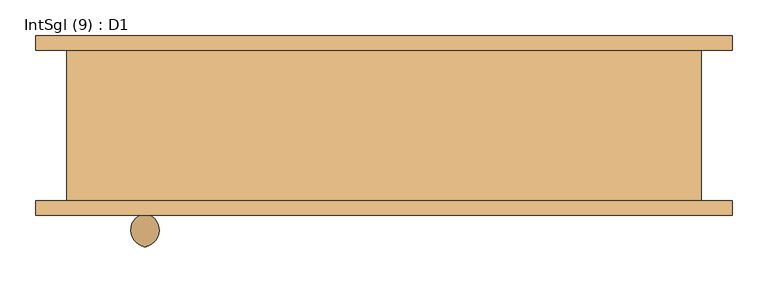
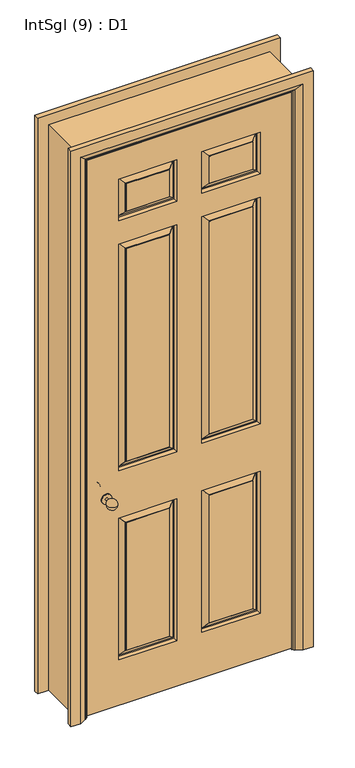
"""IFC4 building model written with IfcOpenShell, lengths in millimetres: door geometry, IntSgl (9) : D1."""

from ifc_helpers import new_model, si_unit, point, frame, origin, place, context, project, spatial, polyline, circle_curve, ellipse_curve, trimmed, outline, extrude, faceted_brep, source, transform, mapped, element, save
from ifc_brep_helpers import plane_surface, cylinder_surface, revolved_surface, advanced_brep


def intsgl_9_d1_ce6ece5b(model_context):
    return source(origin(), model_context, "Body", "SolidModel", [
        advanced_brep(
        [(-328.0, -48.0, 900.0), (-338.0, -48.0, 900.0), (-333.0, -3.562589, 900.0), (-328.0, -63.0, 900.0), (-338.0, -63.0, 900.0), (-353.0, -67.0, 900.0), (-313.0, -67.0, 900.0), (-353.0, -63.0, 900.0), (-313.0, -63.0, 900.0)],
        [
            (0, 1, circle_curve(frame((-333.0, -48.0, 900.0), z_axis=(0.0, 1.0, 0.0), x_axis=(-1.0, 0.0, 0.0)), 5.0)),
            (1, 2, circle_curve(frame((-329.8115138, -26.4213505, 900.0), z_axis=(0.0, 0.0, -1.0), x_axis=(0.0, -1.0, 0.0)), 23.0800654)),
            (2, 0, circle_curve(frame((-336.1884862, -26.4213505, 900.0), z_axis=(0.0, 0.0, -1.0), x_axis=(0.0, -1.0, 0.0)), 23.0800654)),
            (1, 0, circle_curve(frame((-333.0, -48.0, 900.0), z_axis=(0.0, 1.0, 0.0), x_axis=(-1.0, 0.0, 0.0)), 5.0)),
            (0, 3),
            (3, 4, circle_curve(frame((-333.0, -63.0, 900.0), z_axis=(0.0, 1.0, 0.0), x_axis=(-1.0, 0.0, 0.0)), 5.0)),
            (4, 1),
            (4, 3, circle_curve(frame((-333.0, -63.0, 900.0), z_axis=(0.0, 1.0, 0.0), x_axis=(-1.0, 0.0, 0.0)), 5.0)),
            (5, 6, circle_curve(frame((-333.0, -67.0, 900.0), z_axis=(0.0, -1.0, 0.0), x_axis=(1.0, 0.0, 0.0)), 20.0)),
            (6, 5, circle_curve(frame((-333.0, -67.0, 900.0), z_axis=(0.0, -1.0, 0.0), x_axis=(1.0, 0.0, 0.0)), 20.0)),
            (7, 8, circle_curve(frame((-333.0, -63.0, 900.0), z_axis=(0.0, 1.0, 0.0), x_axis=(1.0, 0.0, 0.0)), 20.0)),
            (8, 7, circle_curve(frame((-333.0, -63.0, 900.0), z_axis=(0.0, 1.0, 0.0), x_axis=(1.0, 0.0, 0.0)), 20.0)),
            (5, 7),
            (8, 6),
        ],
        [
            revolved_surface(trimmed(ellipse_curve(frame((-329.8115138, -26.4213505, 900.0), z_axis=(0.0, 0.0, 1.0), x_axis=(0.0, -1.0, 0.0)), 23.0800654, 23.0800654), [point((-333.0, -3.562589, 900.0))], [point((-338.0, -48.0, 900.0))], True, "CARTESIAN"), (-333.0, -63.0, 900.0), (0.0, -1.0, 0.0)),
            cylinder_surface(frame((-333.0, -63.0, 900.0), z_axis=(0.0, -1.0, 0.0), x_axis=(-1.0, 0.0, 0.0)), 5.0),
            plane_surface(frame((-313.0, -67.0, 900.0), z_axis=(0.0, -1.0, 0.0), x_axis=(0.0, 0.0, 1.0))),
            plane_surface(frame((-313.0, -63.0, 900.0), z_axis=(0.0, 1.0, 0.0), x_axis=(0.0, 0.0, -1.0))),
            cylinder_surface(frame((-333.0, -63.0, 900.0), z_axis=(0.0, -1.0, 0.0), x_axis=(1.0, 0.0, 0.0)), 20.0),
        ],
        [
            (0, [[1, 2, 3]]),
            (0, [[-2, 4, -3]]),
            (1, [[-1, 5, 6, 7]]),
            (1, [[-4, -7, 8, -5]]),
            (2, [[9, 10]]),
            (3, [[11, 12], [-6, -8]]),
            (4, [[-9, 13, -12, 14]]),
            (4, [[-10, -14, -11, -13]]),
        ],
    ),
        advanced_brep(
        [(-328.0, -124.0, 900.0), (-333.0, -168.437411, 900.0), (-338.0, -124.0, 900.0), (-338.0, -109.0, 900.0), (-328.0, -109.0, 900.0), (-353.0, -105.0, 900.0), (-313.0, -105.0, 900.0), (-353.0, -109.0, 900.0), (-313.0, -109.0, 900.0)],
        [
            (0, 1, circle_curve(frame((-336.1884862, -145.5786495, 900.0), z_axis=(0.0, 0.0, -1.0), x_axis=(0.0, 1.0, 0.0)), 23.0800654)),
            (1, 2, circle_curve(frame((-329.8115138, -145.5786495, 900.0), z_axis=(0.0, 0.0, -1.0), x_axis=(0.0, 1.0, 0.0)), 23.0800654)),
            (2, 0, circle_curve(frame((-333.0, -124.0, 900.0), z_axis=(0.0, -1.0, 0.0), x_axis=(-1.0, 0.0, 0.0)), 5.0)),
            (0, 2, circle_curve(frame((-333.0, -124.0, 900.0), z_axis=(0.0, -1.0, 0.0), x_axis=(-1.0, 0.0, 0.0)), 5.0)),
            (2, 3),
            (3, 4, circle_curve(frame((-333.0, -109.0, 900.0), z_axis=(0.0, -1.0, 0.0), x_axis=(-1.0, 0.0, 0.0)), 5.0)),
            (4, 0),
            (4, 3, circle_curve(frame((-333.0, -109.0, 900.0), z_axis=(0.0, -1.0, 0.0), x_axis=(-1.0, 0.0, 0.0)), 5.0)),
            (5, 6, circle_curve(frame((-333.0, -105.0, 900.0), z_axis=(0.0, 1.0, 0.0), x_axis=(1.0, 0.0, 0.0)), 20.0)),
            (6, 5, circle_curve(frame((-333.0, -105.0, 900.0), z_axis=(0.0, 1.0, 0.0), x_axis=(1.0, 0.0, 0.0)), 20.0)),
            (7, 8, circle_curve(frame((-333.0, -109.0, 900.0), z_axis=(0.0, -1.0, 0.0), x_axis=(1.0, 0.0, 0.0)), 20.0)),
            (8, 7, circle_curve(frame((-333.0, -109.0, 900.0), z_axis=(0.0, -1.0, 0.0), x_axis=(1.0, 0.0, 0.0)), 20.0)),
            (6, 8),
            (7, 5),
        ],
        [
            revolved_surface(trimmed(ellipse_curve(frame((-329.8115138, -145.5786495, 900.0), z_axis=(0.0, 0.0, -1.0), x_axis=(0.0, 1.0, 0.0)), 23.0800654, 23.0800654), [point((-333.0, -168.437411, 900.0))], [point((-338.0, -124.0, 900.0))], True, "CARTESIAN"), (-333.0, -109.0, 900.0), (0.0, 1.0, 0.0)),
            cylinder_surface(frame((-333.0, -109.0, 900.0), z_axis=(0.0, 1.0, 0.0), x_axis=(-1.0, 0.0, 0.0)), 5.0),
            plane_surface(frame((-313.0, -105.0, 900.0), z_axis=(0.0, 1.0, 0.0), x_axis=(0.0, 0.0, 1.0))),
            plane_surface(frame((-313.0, -109.0, 900.0), z_axis=(0.0, -1.0, 0.0), x_axis=(0.0, 0.0, -1.0))),
            cylinder_surface(frame((-333.0, -109.0, 900.0), z_axis=(0.0, 1.0, 0.0), x_axis=(1.0, 0.0, 0.0)), 20.0),
        ],
        [
            (0, [[1, 2, 3]]),
            (0, [[-1, 4, -2]]),
            (1, [[5, 6, 7, -3]]),
            (1, [[-7, 8, -5, -4]]),
            (2, [[9, 10]]),
            (3, [[11, 12], [-8, -6]]),
            (4, [[13, -11, 14, -10]]),
            (4, [[-14, -12, -13, -9]]),
        ],
    ),
        faceted_brep([(-408.0, -67.0, 2358.0), (408.0, -67.0, 2358.0), (408.0, -67.0, 8.0), (-408.0, -67.0, 8.0), (-50.0, -67.0, 800.0), (-283.0, -67.0, 800.0), (-283.0, -67.0, 200.0), (-50.0, -67.0, 200.0), (283.0, -67.0, 800.0), (50.0, -67.0, 800.0), (50.0, -67.0, 200.0), (283.0, -67.0, 200.0), (-50.0, -67.0, 1958.0), (-283.0, -67.0, 1958.0), (-283.0, -67.0, 1000.0), (-50.0, -67.0, 1000.0), (283.0, -67.0, 1958.0), (50.0, -67.0, 1958.0), (50.0, -67.0, 1000.0), (283.0, -67.0, 1000.0), (-50.0, -67.0, 2233.0), (-283.0, -67.0, 2233.0), (-283.0, -67.0, 2058.0), (-50.0, -67.0, 2058.0), (283.0, -67.0, 2233.0), (50.0, -67.0, 2233.0), (50.0, -67.0, 2058.0), (283.0, -67.0, 2058.0), (-80.0, -67.0, 230.0), (-253.0, -67.0, 230.0), (-253.0, -67.0, 770.0), (-80.0, -67.0, 770.0), (253.0, -67.0, 230.0), (80.0, -67.0, 230.0), (80.0, -67.0, 770.0), (253.0, -67.0, 770.0), (-80.0, -67.0, 1030.0), (-253.0, -67.0, 1030.0), (-253.0, -67.0, 1928.0), (-80.0, -67.0, 1928.0), (253.0, -67.0, 1030.0), (80.0, -67.0, 1030.0), (80.0, -67.0, 1928.0), (253.0, -67.0, 1928.0), (-80.0, -67.0, 2088.0), (-253.0, -67.0, 2088.0), (-253.0, -67.0, 2203.0), (-80.0, -67.0, 2203.0), (253.0, -67.0, 2088.0), (80.0, -67.0, 2088.0), (80.0, -67.0, 2203.0), (253.0, -67.0, 2203.0), (-408.0, -105.0, 2358.0), (-408.0, -105.0, 8.0), (408.0, -105.0, 8.0), (408.0, -105.0, 2358.0), (50.0, -105.0, 800.0), (283.0, -105.0, 800.0), (283.0, -105.0, 200.0), (50.0, -105.0, 200.0), (-283.0, -105.0, 800.0), (-50.0, -105.0, 800.0), (-50.0, -105.0, 200.0), (-283.0, -105.0, 200.0), (50.0, -105.0, 1958.0), (283.0, -105.0, 1958.0), (283.0, -105.0, 1000.0), (50.0, -105.0, 1000.0), (-283.0, -105.0, 1958.0), (-50.0, -105.0, 1958.0), (-50.0, -105.0, 1000.0), (-283.0, -105.0, 1000.0), (50.0, -105.0, 2233.0), (283.0, -105.0, 2233.0), (283.0, -105.0, 2058.0), (50.0, -105.0, 2058.0), (-283.0, -105.0, 2233.0), (-50.0, -105.0, 2233.0), (-50.0, -105.0, 2058.0), (-283.0, -105.0, 2058.0), (80.0, -105.0, 230.0), (253.0, -105.0, 230.0), (253.0, -105.0, 770.0), (80.0, -105.0, 770.0), (-253.0, -105.0, 230.0), (-80.0, -105.0, 230.0), (-80.0, -105.0, 770.0), (-253.0, -105.0, 770.0), (80.0, -105.0, 1030.0), (253.0, -105.0, 1030.0), (253.0, -105.0, 1928.0), (80.0, -105.0, 1928.0), (-253.0, -105.0, 1030.0), (-80.0, -105.0, 1030.0), (-80.0, -105.0, 1928.0), (-253.0, -105.0, 1928.0), (80.0, -105.0, 2088.0), (253.0, -105.0, 2088.0), (253.0, -105.0, 2203.0), (80.0, -105.0, 2203.0), (-253.0, -105.0, 2088.0), (-80.0, -105.0, 2088.0), (-80.0, -105.0, 2203.0), (-253.0, -105.0, 2203.0), (80.0, -104.0, 230.0), (80.0, -104.0, 770.0), (58.0, -90.0, 208.0), (78.0, -104.0, 228.0), (78.0, -104.0, 772.0), (58.0, -90.0, 792.0), (53.0, -90.0, 203.0), (53.0, -90.0, 797.0), (253.0, -104.0, 770.0), (255.0, -104.0, 772.0), (275.0, -90.0, 792.0), (280.0, -90.0, 797.0), (253.0, -104.0, 230.0), (255.0, -104.0, 228.0), (275.0, -90.0, 208.0), (280.0, -90.0, 203.0), (-253.0, -104.0, 230.0), (-253.0, -104.0, 770.0), (-275.0, -90.0, 208.0), (-255.0, -104.0, 228.0), (-255.0, -104.0, 772.0), (-275.0, -90.0, 792.0), (-280.0, -90.0, 203.0), (-280.0, -90.0, 797.0), (-80.0, -104.0, 770.0), (-78.0, -104.0, 772.0), (-58.0, -90.0, 792.0), (-53.0, -90.0, 797.0), (-80.0, -104.0, 230.0), (-78.0, -104.0, 228.0), (-58.0, -90.0, 208.0), (-53.0, -90.0, 203.0), (80.0, -104.0, 1030.0), (80.0, -104.0, 1928.0), (58.0, -90.0, 1008.0), (78.0, -104.0, 1028.0), (78.0, -104.0, 1930.0), (58.0, -90.0, 1950.0), (53.0, -90.0, 1003.0), (53.0, -90.0, 1955.0), (253.0, -104.0, 1928.0), (255.0, -104.0, 1930.0), (275.0, -90.0, 1950.0), (280.0, -90.0, 1955.0), (253.0, -104.0, 1030.0), (255.0, -104.0, 1028.0), (275.0, -90.0, 1008.0), (280.0, -90.0, 1003.0), (-253.0, -104.0, 1030.0), (-253.0, -104.0, 1928.0), (-275.0, -90.0, 1008.0), (-255.0, -104.0, 1028.0), (-255.0, -104.0, 1930.0), (-275.0, -90.0, 1950.0), (-280.0, -90.0, 1003.0), (-280.0, -90.0, 1955.0), (-80.0, -104.0, 1928.0), (-78.0, -104.0, 1930.0), (-58.0, -90.0, 1950.0), (-53.0, -90.0, 1955.0), (-80.0, -104.0, 1030.0), (-78.0, -104.0, 1028.0), (-58.0, -90.0, 1008.0), (-53.0, -90.0, 1003.0), (80.0, -104.0, 2088.0), (80.0, -104.0, 2203.0), (58.0, -90.0, 2066.0), (78.0, -104.0, 2086.0), (78.0, -104.0, 2205.0), (58.0, -90.0, 2225.0), (53.0, -90.0, 2061.0), (53.0, -90.0, 2230.0), (253.0, -104.0, 2203.0), (255.0, -104.0, 2205.0), (275.0, -90.0, 2225.0), (280.0, -90.0, 2230.0), (253.0, -104.0, 2088.0), (255.0, -104.0, 2086.0), (275.0, -90.0, 2066.0), (280.0, -90.0, 2061.0), (-253.0, -104.0, 2088.0), (-253.0, -104.0, 2203.0), (-275.0, -90.0, 2066.0), (-255.0, -104.0, 2086.0), (-255.0, -104.0, 2205.0), (-275.0, -90.0, 2225.0), (-280.0, -90.0, 2061.0), (-280.0, -90.0, 2230.0), (-80.0, -104.0, 2203.0), (-78.0, -104.0, 2205.0), (-58.0, -90.0, 2225.0), (-53.0, -90.0, 2230.0), (-80.0, -104.0, 2088.0), (-78.0, -104.0, 2086.0), (-58.0, -90.0, 2066.0), (-53.0, -90.0, 2061.0), (-80.0, -68.0, 230.0), (-80.0, -68.0, 770.0), (-58.0, -82.0, 208.0), (-78.0, -68.0, 228.0), (-78.0, -68.0, 772.0), (-58.0, -82.0, 792.0), (-53.0, -82.0, 203.0), (-53.0, -82.0, 797.0), (-253.0, -68.0, 770.0), (-255.0, -68.0, 772.0), (-275.0, -82.0, 792.0), (-280.0, -82.0, 797.0), (-253.0, -68.0, 230.0), (-255.0, -68.0, 228.0), (-275.0, -82.0, 208.0), (-280.0, -82.0, 203.0), (253.0, -68.0, 230.0), (253.0, -68.0, 770.0), (275.0, -82.0, 208.0), (255.0, -68.0, 228.0), (255.0, -68.0, 772.0), (275.0, -82.0, 792.0), (280.0, -82.0, 203.0), (280.0, -82.0, 797.0), (80.0, -68.0, 770.0), (78.0, -68.0, 772.0), (58.0, -82.0, 792.0), (53.0, -82.0, 797.0), (80.0, -68.0, 230.0), (78.0, -68.0, 228.0), (58.0, -82.0, 208.0), (53.0, -82.0, 203.0), (-80.0, -68.0, 1030.0), (-80.0, -68.0, 1928.0), (-58.0, -82.0, 1008.0), (-78.0, -68.0, 1028.0), (-78.0, -68.0, 1930.0), (-58.0, -82.0, 1950.0), (-53.0, -82.0, 1003.0), (-53.0, -82.0, 1955.0), (-253.0, -68.0, 1928.0), (-255.0, -68.0, 1930.0), (-275.0, -82.0, 1950.0), (-280.0, -82.0, 1955.0), (-253.0, -68.0, 1030.0), (-255.0, -68.0, 1028.0), (-275.0, -82.0, 1008.0), (-280.0, -82.0, 1003.0), (253.0, -68.0, 1030.0), (253.0, -68.0, 1928.0), (275.0, -82.0, 1008.0), (255.0, -68.0, 1028.0), (255.0, -68.0, 1930.0), (275.0, -82.0, 1950.0), (280.0, -82.0, 1003.0), (280.0, -82.0, 1955.0), (80.0, -68.0, 1928.0), (78.0, -68.0, 1930.0), (58.0, -82.0, 1950.0), (53.0, -82.0, 1955.0), (80.0, -68.0, 1030.0), (78.0, -68.0, 1028.0), (58.0, -82.0, 1008.0), (53.0, -82.0, 1003.0), (-80.0, -68.0, 2088.0), (-80.0, -68.0, 2203.0), (-58.0, -82.0, 2066.0), (-78.0, -68.0, 2086.0), (-78.0, -68.0, 2205.0), (-58.0, -82.0, 2225.0), (-53.0, -82.0, 2061.0), (-53.0, -82.0, 2230.0), (-253.0, -68.0, 2203.0), (-255.0, -68.0, 2205.0), (-275.0, -82.0, 2225.0), (-280.0, -82.0, 2230.0), (-253.0, -68.0, 2088.0), (-255.0, -68.0, 2086.0), (-275.0, -82.0, 2066.0), (-280.0, -82.0, 2061.0), (253.0, -68.0, 2088.0), (253.0, -68.0, 2203.0), (275.0, -82.0, 2066.0), (255.0, -68.0, 2086.0), (255.0, -68.0, 2205.0), (275.0, -82.0, 2225.0), (280.0, -82.0, 2061.0), (280.0, -82.0, 2230.0), (80.0, -68.0, 2203.0), (78.0, -68.0, 2205.0), (58.0, -82.0, 2225.0), (53.0, -82.0, 2230.0), (80.0, -68.0, 2088.0), (78.0, -68.0, 2086.0), (58.0, -82.0, 2066.0), (53.0, -82.0, 2061.0)], [[[0, 1, 2, 3], [4, 5, 6, 7], [8, 9, 10, 11], [12, 13, 14, 15], [16, 17, 18, 19], [20, 21, 22, 23], [24, 25, 26, 27]], [[28, 29, 30, 31]], [[32, 33, 34, 35]], [[36, 37, 38, 39]], [[40, 41, 42, 43]], [[44, 45, 46, 47]], [[48, 49, 50, 51]], [[52, 53, 54, 55], [56, 57, 58, 59], [60, 61, 62, 63], [64, 65, 66, 67], [68, 69, 70, 71], [72, 73, 74, 75], [76, 77, 78, 79]], [[80, 81, 82, 83]], [[84, 85, 86, 87]], [[88, 89, 90, 91]], [[92, 93, 94, 95]], [[96, 97, 98, 99]], [[100, 101, 102, 103]], [[3, 53, 52, 0]], [[2, 54, 53, 3]], [[1, 55, 54, 2]], [[0, 52, 55, 1]], [[104, 80, 83, 105]], [[106, 107, 108, 109]], [[56, 59, 110, 111]], [[83, 82, 112, 105]], [[108, 113, 114, 109]], [[111, 115, 57, 56]], [[82, 81, 116, 112]], [[113, 117, 118, 114]], [[115, 119, 58, 57]], [[104, 116, 81, 80]], [[107, 117, 113, 108], [105, 112, 116, 104]], [[106, 118, 117, 107]], [[110, 119, 115, 111], [109, 114, 118, 106]], [[59, 58, 119, 110]], [[120, 84, 87, 121]], [[122, 123, 124, 125]], [[60, 63, 126, 127]], [[87, 86, 128, 121]], [[124, 129, 130, 125]], [[127, 131, 61, 60]], [[86, 85, 132, 128]], [[129, 133, 134, 130]], [[131, 135, 62, 61]], [[120, 132, 85, 84]], [[123, 133, 129, 124], [121, 128, 132, 120]], [[122, 134, 133, 123]], [[126, 135, 131, 127], [125, 130, 134, 122]], [[63, 62, 135, 126]], [[136, 88, 91, 137]], [[138, 139, 140, 141]], [[64, 67, 142, 143]], [[91, 90, 144, 137]], [[140, 145, 146, 141]], [[143, 147, 65, 64]], [[90, 89, 148, 144]], [[145, 149, 150, 146]], [[147, 151, 66, 65]], [[136, 148, 89, 88]], [[139, 149, 145, 140], [137, 144, 148, 136]], [[138, 150, 149, 139]], [[142, 151, 147, 143], [141, 146, 150, 138]], [[67, 66, 151, 142]], [[152, 92, 95, 153]], [[154, 155, 156, 157]], [[68, 71, 158, 159]], [[95, 94, 160, 153]], [[156, 161, 162, 157]], [[159, 163, 69, 68]], [[94, 93, 164, 160]], [[161, 165, 166, 162]], [[163, 167, 70, 69]], [[152, 164, 93, 92]], [[155, 165, 161, 156], [153, 160, 164, 152]], [[154, 166, 165, 155]], [[158, 167, 163, 159], [157, 162, 166, 154]], [[71, 70, 167, 158]], [[168, 96, 99, 169]], [[170, 171, 172, 173]], [[72, 75, 174, 175]], [[99, 98, 176, 169]], [[172, 177, 178, 173]], [[175, 179, 73, 72]], [[98, 97, 180, 176]], [[177, 181, 182, 178]], [[179, 183, 74, 73]], [[168, 180, 97, 96]], [[171, 181, 177, 172], [169, 176, 180, 168]], [[170, 182, 181, 171]], [[174, 183, 179, 175], [173, 178, 182, 170]], [[75, 74, 183, 174]], [[184, 100, 103, 185]], [[186, 187, 188, 189]], [[76, 79, 190, 191]], [[103, 102, 192, 185]], [[188, 193, 194, 189]], [[191, 195, 77, 76]], [[102, 101, 196, 192]], [[193, 197, 198, 194]], [[195, 199, 78, 77]], [[184, 196, 101, 100]], [[187, 197, 193, 188], [185, 192, 196, 184]], [[186, 198, 197, 187]], [[190, 199, 195, 191], [189, 194, 198, 186]], [[79, 78, 199, 190]], [[200, 28, 31, 201]], [[202, 203, 204, 205]], [[4, 7, 206, 207]], [[31, 30, 208, 201]], [[204, 209, 210, 205]], [[207, 211, 5, 4]], [[30, 29, 212, 208]], [[209, 213, 214, 210]], [[211, 215, 6, 5]], [[200, 212, 29, 28]], [[203, 213, 209, 204], [201, 208, 212, 200]], [[202, 214, 213, 203]], [[206, 215, 211, 207], [205, 210, 214, 202]], [[7, 6, 215, 206]], [[216, 32, 35, 217]], [[218, 219, 220, 221]], [[8, 11, 222, 223]], [[35, 34, 224, 217]], [[220, 225, 226, 221]], [[223, 227, 9, 8]], [[34, 33, 228, 224]], [[225, 229, 230, 226]], [[227, 231, 10, 9]], [[216, 228, 33, 32]], [[219, 229, 225, 220], [217, 224, 228, 216]], [[218, 230, 229, 219]], [[222, 231, 227, 223], [221, 226, 230, 218]], [[11, 10, 231, 222]], [[232, 36, 39, 233]], [[234, 235, 236, 237]], [[12, 15, 238, 239]], [[39, 38, 240, 233]], [[236, 241, 242, 237]], [[239, 243, 13, 12]], [[38, 37, 244, 240]], [[241, 245, 246, 242]], [[243, 247, 14, 13]], [[232, 244, 37, 36]], [[235, 245, 241, 236], [233, 240, 244, 232]], [[234, 246, 245, 235]], [[238, 247, 243, 239], [237, 242, 246, 234]], [[15, 14, 247, 238]], [[248, 40, 43, 249]], [[250, 251, 252, 253]], [[16, 19, 254, 255]], [[43, 42, 256, 249]], [[252, 257, 258, 253]], [[255, 259, 17, 16]], [[42, 41, 260, 256]], [[257, 261, 262, 258]], [[259, 263, 18, 17]], [[248, 260, 41, 40]], [[251, 261, 257, 252], [249, 256, 260, 248]], [[250, 262, 261, 251]], [[254, 263, 259, 255], [253, 258, 262, 250]], [[19, 18, 263, 254]], [[264, 44, 47, 265]], [[266, 267, 268, 269]], [[20, 23, 270, 271]], [[47, 46, 272, 265]], [[268, 273, 274, 269]], [[271, 275, 21, 20]], [[46, 45, 276, 272]], [[273, 277, 278, 274]], [[275, 279, 22, 21]], [[264, 276, 45, 44]], [[267, 277, 273, 268], [265, 272, 276, 264]], [[266, 278, 277, 267]], [[270, 279, 275, 271], [269, 274, 278, 266]], [[23, 22, 279, 270]], [[280, 48, 51, 281]], [[282, 283, 284, 285]], [[24, 27, 286, 287]], [[51, 50, 288, 281]], [[284, 289, 290, 285]], [[287, 291, 25, 24]], [[50, 49, 292, 288]], [[289, 293, 294, 290]], [[291, 295, 26, 25]], [[280, 292, 49, 48]], [[283, 293, 289, 284], [281, 288, 292, 280]], [[282, 294, 293, 283]], [[286, 295, 291, 287], [285, 290, 294, 282]], [[27, 26, 295, 286]]]),
        faceted_brep([(-410.0, -105.0, 0.0), (-442.0, -105.0, 0.0), (-442.0, 105.0, 0.0), (-410.0, 105.0, 0.0), (-410.0, 105.0, 2360.0), (-410.0, -105.0, 2360.0), (-442.0, 105.0, 2392.0), (-442.0, -105.0, 2392.0), (410.0, -105.0, 0.0), (410.0, 105.0, 0.0), (442.0, 105.0, 0.0), (442.0, -105.0, 0.0), (410.0, -105.0, 2360.0), (442.0, -105.0, 2392.0), (442.0, 105.0, 2392.0), (410.0, 105.0, 2360.0)], [[[0, 1, 2, 3]], [[3, 4, 5, 0]], [[2, 6, 4, 3]], [[1, 7, 6, 2]], [[0, 5, 7, 1]], [[8, 9, 10, 11]], [[12, 8, 11, 13]], [[13, 11, 10, 14]], [[14, 10, 9, 15]], [[15, 9, 8, 12]], [[4, 15, 12, 5]], [[6, 14, 15, 4]], [[7, 13, 14, 6]], [[5, 12, 13, 7]]]),
        extrude(outline(polyline([(0.0, -391.0), (2341.0, -391.0), (2341.0, 391.0), (0.0, 391.0), (0.0, 410.0), (2360.0, 410.0), (2360.0, -410.0), (0.0, -410.0), (0.0, -391.0)])), frame((0.0, -65.0, 0.0), z_axis=(0.0, 1.0, 0.0), x_axis=(0.0, 0.0, 1.0)), (0.0, 0.0, 1.0), 32.0),
        advanced_brep(
        [(-485.0, 125.0, 0.0), (-445.0, 125.0, 0.0), (-419.0, 111.0, 0.0), (-415.0, 105.0, 0.0), (-485.0, 105.0, 0.0), (-485.0, 105.0, 2435.0), (-485.0, 125.0, 2435.0), (-415.0, 105.0, 2365.0), (415.0, 105.0, 2365.0), (415.0, 105.0, 0.0), (485.0, 105.0, 0.0), (485.0, 105.0, 2435.0), (-419.0, 111.0, 2369.0), (-445.0, 125.0, 2395.0), (485.0, 125.0, 2435.0), (485.0, 125.0, 0.0), (445.0, 125.0, 0.0), (445.0, 125.0, 2395.0), (419.0, 111.0, 0.0), (419.0, 111.0, 2369.0)],
        [
            (0, 1),
            (1, 2),
            (2, 3, circle_curve(frame((-423.0, 104.0, 0.0), z_axis=(0.0, 0.0, -1.0), x_axis=(-1.0, 0.0, 0.0)), 8.0622577)),
            (3, 4),
            (4, 0),
            (4, 5),
            (5, 6),
            (6, 0),
            (3, 7),
            (7, 8),
            (8, 9),
            (9, 10),
            (10, 11),
            (11, 5),
            (2, 12),
            (12, 7, ellipse_curve(frame((-423.0, 104.0, 2373.0), z_axis=(-0.7071067811865475, 0.0, -0.7071067811865475), x_axis=(0.7071067811865474, 0.0, -0.7071067811865476)), 11.4017543, 8.0622577)),
            (1, 13),
            (13, 12),
            (6, 14),
            (14, 15),
            (15, 16),
            (16, 17),
            (17, 13),
            (10, 15),
            (14, 11),
            (9, 18, circle_curve(frame((423.0, 104.0, 0.0), z_axis=(0.0, 0.0, -1.0), x_axis=(1.0, 0.0, 0.0)), 8.0622577)),
            (18, 16),
            (19, 18),
            (8, 19, ellipse_curve(frame((423.0, 104.0, 2373.0), z_axis=(0.7071067811865475, 0.0, -0.7071067811865475), x_axis=(0.7071067811865474, 0.0, 0.7071067811865476)), 11.4017543, 8.0622577)),
            (19, 17),
            (12, 19),
        ],
        [
            plane_surface(frame((-415.0, 105.0, 0.0), z_axis=(0.0, 0.0, -1.0), x_axis=(0.0, 1.0, 0.0))),
            plane_surface(frame((-485.0, 125.0, 0.0), z_axis=(-1.0, 0.0, 0.0), x_axis=(0.0, 0.0, 1.0))),
            plane_surface(frame((-485.0, 105.0, 0.0), z_axis=(0.0, -1.0, 0.0), x_axis=(0.0, 0.0, 1.0))),
            cylinder_surface(frame((-423.0, 104.0, 0.0), z_axis=(0.0, 0.0, -1.0), x_axis=(-1.0, 0.0, 0.0)), 8.0622577),
            plane_surface(frame((-419.0, 111.0, 0.0), z_axis=(0.4740998230350183, 0.8804710999221749, 0.0), x_axis=(0.0, 0.0, 1.0))),
            plane_surface(frame((-445.0, 125.0, 0.0), z_axis=(0.0, 1.0, 0.0), x_axis=(0.0, 0.0, 1.0))),
            plane_surface(frame((485.0, 125.0, 2435.0), z_axis=(1.0, 0.0, 0.0), x_axis=(0.0, 0.0, -1.0))),
            plane_surface(frame((415.0, 105.0, 0.0), z_axis=(0.0, 0.0, -1.0), x_axis=(0.0, 1.0, 0.0))),
            cylinder_surface(frame((423.0, 104.0, 2365.0), z_axis=(0.0, 0.0, 1.0), x_axis=(1.0, 0.0, 0.0)), 8.0622577),
            plane_surface(frame((419.0, 111.0, 2369.0), z_axis=(-0.4740998230350183, 0.8804710999221749, 0.0), x_axis=(0.0, 0.0, -1.0))),
            plane_surface(frame((-485.0, 125.0, 2435.0), z_axis=(0.0, 0.0, 1.0), x_axis=(1.0, 0.0, 0.0))),
            cylinder_surface(frame((-415.0, 104.0, 2373.0), z_axis=(-1.0, 0.0, 0.0), x_axis=(0.0, 0.0, 1.0)), 8.0622577),
            plane_surface(frame((-419.0, 111.0, 2369.0), z_axis=(0.0, 0.8804710999221749, -0.4740998230350183), x_axis=(1.0, 0.0, 0.0))),
        ],
        [
            (0, [[1, 2, 3, 4, 5]]),
            (1, [[6, 7, 8, -5]]),
            (2, [[9, 10, 11, 12, 13, 14, -6, -4]]),
            (3, [[15, 16, -9, -3]]),
            (4, [[17, 18, -15, -2]]),
            (5, [[-8, 19, 20, 21, 22, 23, -17, -1]]),
            (6, [[-13, 24, -20, 25]]),
            (7, [[-24, -12, 26, 27, -21]]),
            (8, [[28, -26, -11, 29]]),
            (9, [[-22, -27, -28, 30]]),
            (10, [[-14, -25, -19, -7]]),
            (11, [[31, -29, -10, -16]]),
            (12, [[-23, -30, -31, -18]]),
        ],
    ),
        advanced_brep(
        [(485.0, -125.0, 0.0), (445.0, -125.0, 0.0), (419.0, -111.0, 0.0), (415.0, -105.0, 0.0), (485.0, -105.0, 0.0), (485.0, -105.0, 2435.0), (485.0, -125.0, 2435.0), (415.0, -105.0, 2365.0), (-415.0, -105.0, 2365.0), (-415.0, -105.0, 0.0), (-485.0, -105.0, 0.0), (-485.0, -105.0, 2435.0), (419.0, -111.0, 2369.0), (445.0, -125.0, 2395.0), (-485.0, -125.0, 2435.0), (-485.0, -125.0, 0.0), (-445.0, -125.0, 0.0), (-445.0, -125.0, 2395.0), (-419.0, -111.0, 0.0), (-419.0, -111.0, 2369.0)],
        [
            (0, 1),
            (1, 2),
            (2, 3, circle_curve(frame((423.0, -104.0, 0.0), z_axis=(0.0, 0.0, -1.0), x_axis=(1.0, 0.0, 0.0)), 8.0622577)),
            (3, 4),
            (4, 0),
            (4, 5),
            (5, 6),
            (6, 0),
            (3, 7),
            (7, 8),
            (8, 9),
            (9, 10),
            (10, 11),
            (11, 5),
            (2, 12),
            (12, 7, ellipse_curve(frame((423.0, -104.0, 2373.0), z_axis=(0.7071067811865475, 0.0, -0.7071067811865475), x_axis=(-0.7071067811865474, 0.0, -0.7071067811865476)), 11.4017543, 8.0622577)),
            (1, 13),
            (13, 12),
            (6, 14),
            (14, 15),
            (15, 16),
            (16, 17),
            (17, 13),
            (10, 15),
            (14, 11),
            (9, 18, circle_curve(frame((-423.0, -104.0, 0.0), z_axis=(0.0, 0.0, -1.0), x_axis=(-1.0, 0.0, 0.0)), 8.0622577)),
            (18, 16),
            (19, 18),
            (8, 19, ellipse_curve(frame((-423.0, -104.0, 2373.0), z_axis=(-0.7071067811865475, 0.0, -0.7071067811865475), x_axis=(-0.7071067811865474, 0.0, 0.7071067811865476)), 11.4017543, 8.0622577)),
            (19, 17),
            (12, 19),
        ],
        [
            plane_surface(frame((415.0, -105.0, 0.0), z_axis=(0.0, 0.0, -1.0), x_axis=(0.0, -1.0, 0.0))),
            plane_surface(frame((485.0, -125.0, 0.0), z_axis=(1.0, 0.0, 0.0), x_axis=(0.0, 0.0, 1.0))),
            plane_surface(frame((485.0, -105.0, 0.0), z_axis=(0.0, 1.0, 0.0), x_axis=(0.0, 0.0, 1.0))),
            cylinder_surface(frame((423.0, -104.0, 0.0), z_axis=(0.0, 0.0, -1.0), x_axis=(1.0, 0.0, 0.0)), 8.0622577),
            plane_surface(frame((419.0, -111.0, 0.0), z_axis=(-0.4740998230350183, -0.8804710999221749, 0.0), x_axis=(0.0, 0.0, 1.0))),
            plane_surface(frame((445.0, -125.0, 0.0), z_axis=(0.0, -1.0, 0.0), x_axis=(0.0, 0.0, 1.0))),
            plane_surface(frame((-485.0, -125.0, 2435.0), z_axis=(-1.0, 0.0, 0.0), x_axis=(0.0, 0.0, -1.0))),
            plane_surface(frame((-415.0, -105.0, 0.0), z_axis=(0.0, 0.0, -1.0), x_axis=(0.0, -1.0, 0.0))),
            cylinder_surface(frame((-423.0, -104.0, 2365.0), z_axis=(0.0, 0.0, 1.0), x_axis=(-1.0, 0.0, 0.0)), 8.0622577),
            plane_surface(frame((-419.0, -111.0, 2369.0), z_axis=(0.4740998230350183, -0.8804710999221749, 0.0), x_axis=(0.0, 0.0, -1.0))),
            plane_surface(frame((485.0, -125.0, 2435.0), z_axis=(0.0, 0.0, 1.0), x_axis=(-1.0, 0.0, 0.0))),
            cylinder_surface(frame((415.0, -104.0, 2373.0), z_axis=(1.0, 0.0, 0.0), x_axis=(0.0, 0.0, 1.0)), 8.0622577),
            plane_surface(frame((419.0, -111.0, 2369.0), z_axis=(0.0, -0.8804710999221749, -0.4740998230350183), x_axis=(-1.0, 0.0, 0.0))),
        ],
        [
            (0, [[1, 2, 3, 4, 5]]),
            (1, [[6, 7, 8, -5]]),
            (2, [[9, 10, 11, 12, 13, 14, -6, -4]]),
            (3, [[15, 16, -9, -3]]),
            (4, [[17, 18, -15, -2]]),
            (5, [[-8, 19, 20, 21, 22, 23, -17, -1]]),
            (6, [[-13, 24, -20, 25]]),
            (7, [[-24, -12, 26, 27, -21]]),
            (8, [[28, -26, -11, 29]]),
            (9, [[-22, -27, -28, 30]]),
            (10, [[-14, -25, -19, -7]]),
            (11, [[31, -29, -10, -16]]),
            (12, [[-23, -30, -31, -18]]),
        ],
    ),
    ])


if __name__ == "__main__":
    model = new_model("IFC4")
    model_context = context("Model", 3, world=origin())
    ifc_project = project(units=[si_unit("LENGTHUNIT", "METRE", prefix="MILLI")], contexts=[model_context])
    site = spatial("IfcSite", under=ifc_project)
    building = spatial("IfcBuilding", under=site)
    placement = place(None, origin())
    intsgl_9_d1_shape = intsgl_9_d1_ce6ece5b(model_context)
    element("IfcDoor", 1, ObjectType="IntSgl (9) : D1", at=placement, inside=building, context=model_context, shape_type="MappedRepresentation", body=[
        mapped(intsgl_9_d1_shape, transform((0.0, 0.0, 0.0), x_axis=(1.0, 0.0, 0.0), y_axis=(0.0, 1.0, 0.0), z_axis=(0.0, 0.0, 1.0))),
    ])
    save(model, "model.ifc")

# Revit data of these elements
# Type "IntSgl (9) : D1"
#   Type Mark = "49"
#   Operation = "SingleSwingRight"
#   Manufacturer = "Revit"
#   Keynote = "L20"
#   UnderCut = 8 mm
#   Tolerance = 2 mm
#   Thickness = 38 mm
#   Structural Tolerance = 8 mm
#   StopDepth = 32 mm
#   Stop Thickness = 19 mm
#   Stile Top Rail = 125 mm
#   Stile Shutting = 125 mm
#   Stile Muntin Rail = 100 mm
#   Stile Lock Rail = 200 mm
#   Stile Intermediate/Frieze = 100 mm
#   Stile Hanging = 125 mm
#   Stile Bottom Rail = 200 mm
#   Rough Width = 900 mm
#   Rough Height = 2400 mm
#   Height to Top Lock Rail = 1000 mm
#   Handle Z Distance = 900 mm
#   Handle X Distance = 75 mm
#   Frame Thickness = 32 mm
#   Door Panel Width = 816 mm
#   Height = 2400 mm
#   Width = 900 mm
#   Door Panel Thickness = 38 mm
#   Door Panel Offset = 0 mm
#   Door Panel Height = 2350 mm
#   Architrave Setback = 5 mm
#   Vis - Ironmongery = yes
#   Material Ironmongery = Door - Handle
#   Material Frame = Door - Frame/Mullion
#   Material Door = Door - Panel
#   Material Architrave = Door - Architrave
#   Function = (empty or 0)
#   Wall Closure = (empty or 0)
# Element 1 (IfcDoor, "IntSgl (9) : D1")
#   Materials on its faces: "Door - Panel", "Door - Architrave", "Door - Frame/Mullion", "Door - Handle"
# Materials
#   "Door - Handle": colour RGB 0 0 0, transparency 0, Keynote = "P21", Cost = 0, Export to IFC = 0
#   "Door - Frame/Mullion": class "Wood", colour RGB 212 179 113, transparency 0, Keynote = "L20", Cost = 0, Export to IFC = 0
#   "Door - Panel": class "Wood", colour RGB 210 159 95, transparency 0, Keynote = "L20", Cost = 0, Export to IFC = 0
#   "Door - Architrave": class "Wood", colour RGB 154 90 5, transparency 0, Keynote = "P20", Cost = 0, Export to IFC = 0
